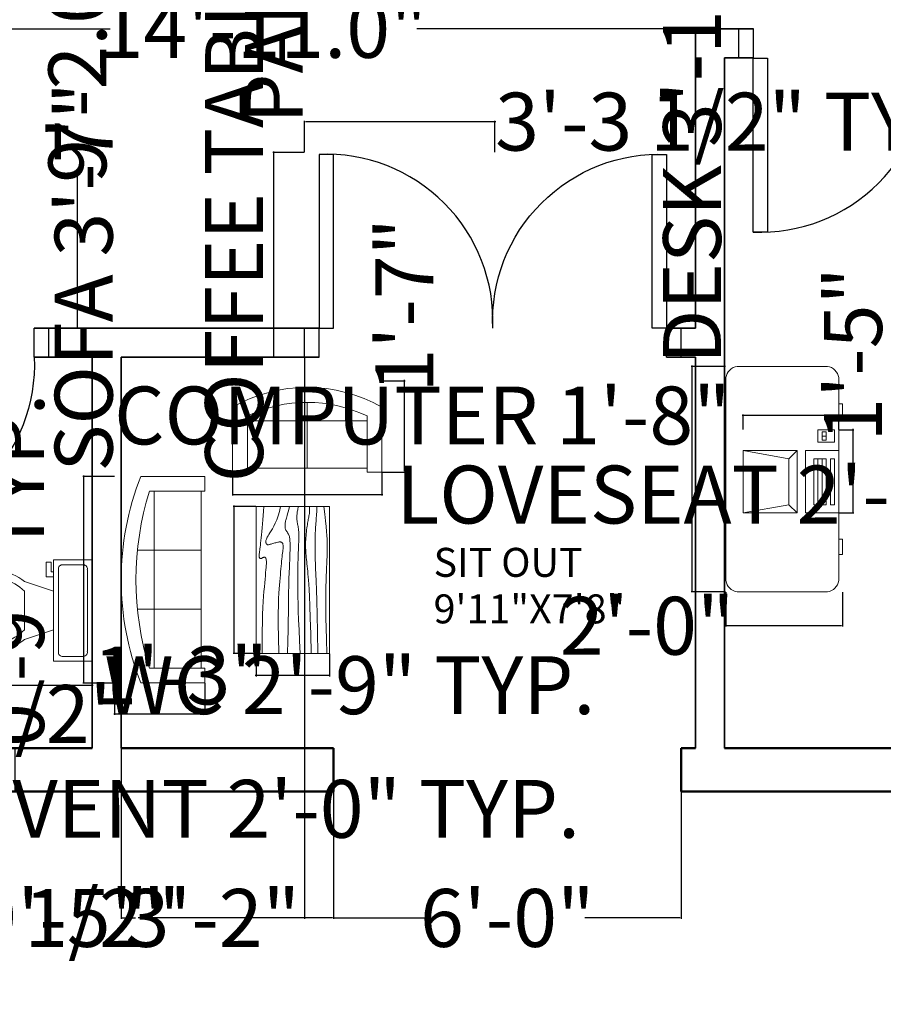
# Model space of a CAD drawing. Units: inches. Extents: x -52 to 472, y -40 to 644.
# Tile 2 of 6: x 71 to 250, y -40 to 164. Entities that reach past the tile are written whole.
import ezdxf

# ---------------------------------------------------------------- set-up
doc = ezdxf.new("R2010")
doc.units = ezdxf.units.IN
doc.header["$MEASUREMENT"] = 0
for name, color, linetype, lineweight in [('A-ANNO-DIMS', 7, 'Continuous', 13), ('A-ANNO-TEXT', 7, 'Continuous', 18), ('A-EQPM', 8, 'Continuous', 13), ('DOORS', 2, 'Continuous', 25), ('FURNITURE', 6, 'Continuous', 13), ('INNER WALL', 1, 'Continuous', 35), ('OUTER WALL', 1, 'Continuous', 50), ('S-PLUM', 151, 'Continuous', 18)]:
    doc.layers.add(name, color=color, linetype=linetype, lineweight=lineweight)
doc.styles.get("Standard").update_dxf_attribs({"font": 'arial.ttf'})
doc.dimstyles.get("Standard").update_dxf_attribs({"dimtxt": 12, "dimasz": 0.18, "dimexe": 0.18, "dimexo": 0.0625, "dimgap": 0.09, "dimtad": 0, "dimdec": 1, "dimzin": 0, "dimdsep": 46, "dimlunit": 3, "dimtxsty": 'Standard', "dimcen": 0.09, "dimadec": 0, "dimazin": 0, "dimtfac": 1, "dimtdec": 1, "dimtofl": 0, "dimtmove": 0, "dimatfit": 3, "dimfxl": 1, "dimtolj": 1, "dimtzin": 0, "dimarcsym": 0})

# ---------------------------------------------------------------- blocks, each defined once
blk = doc.blocks.new('Sofa - Roundback Loveseat 5 ft.')
for p, q in [((0, -32.44198), (0, -5.99998)), ((-24, -33.99998), (-24, -11.46958)), ((24.00004, -33.99998), (24.00004, -11.46958)), ((-23.9998, -13.38178), (23.99986, -13.38178)), ((-24, -32.44198), (24.00004, -32.44198))]:
    blk.add_line(p, q)
for points in [[(-24, -33.99998), (-30, -33.99998), (-30, -7.99998)], [(30.00004, -7.99998), (30.00004, -33.99998), (24.00004, -33.99998)]]:
    blk.add_lwpolyline(points)
for centre, radius, start, end in [((0, -60.24998), 60.24998, 60.13715, 119.8628), ((0, -61.38438), 55.38444, 64.32083, 115.6792)]:
    blk.add_arc(centre, radius, start, end)
blk = doc.blocks.new('Sofa - Roundback 7 ft.')
for p, q in [((-12.00002, -32.4421), (-12.00003, -6.5971)), ((11.99997, -32.4421), (11.99998, -6.5971)), ((-36.000027, -34), (-36.000027, -11.4696)), ((35.99998, -34), (35.99998, -11.4696)), ((-35.999844, -13.3819), (35.9998, -13.3819)), ((-36.000027, -32.4421), (35.99998, -32.4421))]:
    blk.add_line(p, q)
for points in [[(-36.000027, -34), (-42.000027, -34), (-42.000027, -8)], [(41.99998, -8), (41.99998, -34), (35.99998, -34)]]:
    blk.add_lwpolyline(points)
for centre, radius, start, end in [((0, -114.25), 114.25, 68.43141, 111.5686), ((-0.00001, -127.1968), 121.1968, 72.72033, 107.2797)]:
    blk.add_arc(centre, radius, start, end)
blk = doc.blocks.new('Table - Rectangular Woodgrain 60 x 30 in.')
for p, q in [((0, 0), (0, -30)), ((60, 0), (0, 0)), ((60, -30), (60, 0)), ((0, -30), (60, -30))]:
    blk.add_line(p, q)
for points in [[(0, -2.4), (4.8155, -2.418), (9.0302, -2.4688), (12.709, -2.5477), (15.9167, -2.65), (18.7181, -2.7711), (21.1781, -2.9063), (23.3616, -3.0508), (25.3333, -3.2), (27.1477, -3.3495), (28.8172, -3.4958), (30.3437, -3.636), (31.7291, -3.7667), (32.9756, -3.8849), (34.0849, -3.9875), (35.059, -4.0714), (35.9, -4.1334), (36.6114, -4.1711), (37.2041, -4.1854), (37.6906, -4.1779), (38.0833, -4.15), (38.3948, -4.1034), (38.6375, -4.0396), (38.8239, -3.9602), (38.9666, -3.8667), (39.0764, -3.7608), (39.1573, -3.6448), (39.2116, -3.521), (39.2416, -3.3917), (39.2498, -3.2593), (39.2385, -3.1261), (39.21, -2.9944), (39.1666, -2.8667), (39.111, -2.7447), (39.0468, -2.6281), (38.978, -2.5163), (38.9083, -2.4083), (38.8418, -2.3035), (38.7823, -2.201), (38.7337, -2.1001), (38.7, -2), (38.6844, -1.9003), (38.6875, -1.8021), (38.7094, -1.707), (38.75, -1.6167), (38.8094, -1.5326), (38.8875, -1.4563), (38.9844, -1.3893), (39.1, -1.3333), (39.2351, -1.2896), (39.3937, -1.2583), (39.5804, -1.2396), (39.8, -1.2333), (40.057, -1.2396), (40.3562, -1.2583), (40.7023, -1.2896), (41.1, -1.3333), (41.5547, -1.3895), (42.0755, -1.4573), (42.6721, -1.5361), (43.3542, -1.625), (44.1316, -1.7233), (45.014, -1.8302), (46.0114, -1.9449), (47.1333, -2.0667), (48.3862, -2.1947), (49.7625, -2.3281), (51.2513, -2.4663), (52.8416, -2.6083), (54.5226, -2.7535), (56.2833, -2.9011), (58.1127, -3.0501), (60, -3.2)], [(0, -9.2), (6.5759, -9.0858), (11.9385, -9.0365), (16.2527, -9.0418), (19.6833, -9.0917), (22.3952, -9.1759), (24.5531, -9.2844), (26.322, -9.4069), (27.8666, -9.5333), (29.3241, -9.6553), (30.7203, -9.7719), (32.0532, -9.8837), (33.3208, -9.9917), (34.5213, -10.0965), (35.6526, -10.199), (36.7128, -10.2999), (37.7, -10.4), (38.6129, -10.4996), (39.4531, -10.5969), (40.223, -10.6895), (40.925, -10.775), (41.5613, -10.8512), (42.1344, -10.9156), (42.6465, -10.966), (43.1, -11), (43.4976, -11.0158), (43.8437, -11.0136), (44.143, -10.9942), (44.4, -10.9583), (44.6195, -10.9069), (44.8062, -10.8406), (44.9648, -10.7603), (45.1, -10.6667), (45.2155, -10.5598), (45.3114, -10.4365), (45.3871, -10.2929), (45.4416, -10.125), (45.4743, -9.929), (45.4844, -9.7011), (45.4709, -9.4371), (45.4333, -9.1333), (45.3716, -8.7883), (45.2896, -8.4104), (45.1919, -8.0107), (45.0833, -7.6), (44.9685, -7.1893), (44.8521, -6.7896), (44.7388, -6.4117), (44.6333, -6.0667), (44.54, -5.7628), (44.4614, -5.4979), (44.4001, -5.2675), (44.3583, -5.0667), (44.3384, -4.8909), (44.3427, -4.7354), (44.3736, -4.5956), (44.4333, -4.4667), (44.5236, -4.3453), (44.6427, -4.2333), (44.7884, -4.1339), (44.9583, -4.05), (45.1501, -3.9849), (45.3614, -3.9417), (45.59, -3.9234), (45.8333, -3.9333), (46.0915, -3.9749), (46.3734, -4.0531), (46.6906, -4.1736), (47.0542, -4.3417), (47.4756, -4.5629), (47.9661, -4.8427), (48.5372, -5.1866), (49.2, -5.6), (49.9676, -6.0844), (50.8594, -6.625), (51.8965, -7.2031), (53.1, -7.8), (54.491, -8.3969), (56.0906, -8.975), (57.9199, -9.5156), (60, -10)], [(0, -12.8), (5.1847, -12.9322), (9.6213, -13.0323), (13.3963, -13.1059), (16.5958, -13.1583), (19.3063, -13.1952), (21.614, -13.2219), (23.6054, -13.2439), (25.3666, -13.2667), (26.9728, -13.2947), (28.4531, -13.3281), (29.8256, -13.3663), (31.1083, -13.4083), (32.3191, -13.4535), (33.476, -13.501), (34.597, -13.5501), (35.7, -13.6), (36.7984, -13.6497), (37.8875, -13.6979), (38.9578, -13.743), (40, -13.7833), (41.0047, -13.8174), (41.9625, -13.8438), (42.864, -13.8607), (43.7, -13.8667), (44.4631, -13.8604), (45.1552, -13.8417), (45.7801, -13.8104), (46.3416, -13.7667), (46.8439, -13.7104), (47.2906, -13.6417), (47.6858, -13.5604), (48.0333, -13.4667), (48.3375, -13.3608), (48.6042, -13.2448), (48.8396, -13.121), (49.05, -12.9917), (49.2417, -12.8593), (49.4208, -12.7261), (49.5937, -12.5944), (49.7667, -12.4667), (49.9452, -12.3451), (50.1323, -12.2313), (50.3303, -12.1268), (50.5416, -12.0333), (50.7686, -11.9524), (51.0135, -11.8854), (51.2788, -11.8341), (51.5666, -11.8), (51.8785, -11.7843), (52.2116, -11.7865), (52.562, -11.8059), (52.926, -11.8417), (53.2998, -11.8931), (53.6795, -11.9594), (54.0614, -12.0397), (54.4416, -12.1333), (54.8223, -12.2401), (55.2293, -12.3625), (55.6942, -12.5037), (56.2489, -12.6667), (56.9251, -12.8547), (57.7545, -13.0708), (58.7689, -13.3182), (60, -13.6)], [(0, -18), (5.124, -17.7273), (9.6609, -17.5057), (13.6705, -17.3303), (17.2125, -17.1958), (20.3467, -17.0973), (23.1328, -17.0297), (25.6307, -16.9878), (27.9, -16.9667), (29.9928, -16.9617), (31.9302, -16.9703), (33.7254, -16.9907), (35.3917, -17.0208), (36.9423, -17.0588), (38.3906, -17.1026), (39.7499, -17.1503), (41.0333, -17.2), (42.2519, -17.2496), (43.4073, -17.2969), (44.4986, -17.3395), (45.525, -17.375), (46.4858, -17.4012), (47.3802, -17.4156), (48.2074, -17.416), (48.9667, -17.4), (49.6583, -17.3662), (50.2872, -17.3167), (50.8595, -17.2547), (51.3812, -17.1833), (51.8584, -17.1057), (52.2971, -17.025), (52.7034, -16.9443), (53.0833, -16.8667), (53.443, -16.7951), (53.789, -16.7313), (54.128, -16.6768), (54.4666, -16.6334), (54.8115, -16.6024), (55.1693, -16.5854), (55.5465, -16.5841), (55.95, -16.6), (56.3828, -16.6337), (56.8346, -16.6823), (57.2915, -16.7418), (57.7396, -16.8084), (58.165, -16.878), (58.5539, -16.9469), (58.8924, -17.0111), (59.1666, -17.0667), (59.3679, -17.1107), (59.5078, -17.1438), (59.6032, -17.1675), (59.6708, -17.1833), (59.7275, -17.193), (59.7901, -17.1979), (59.8753, -17.1998), (60, -17.2)], [(0, -22.4), (8.0098, -22.2501), (14.4094, -22.1011), (19.4168, -21.9535), (23.25, -21.8083), (26.1269, -21.6663), (28.2656, -21.5281), (29.884, -21.3947), (31.2, -21.2667), (32.3967, -21.1448), (33.5172, -21.0292), (34.5697, -20.9198), (35.5625, -20.8167), (36.5037, -20.7198), (37.4015, -20.6292), (38.2642, -20.5448), (39.1, -20.4667), (39.9164, -20.3951), (40.7187, -20.3313), (41.5117, -20.2768), (42.3, -20.2333), (43.0883, -20.2024), (43.8812, -20.1854), (44.6836, -20.1841), (45.5, -20.2), (46.3328, -20.234), (47.1747, -20.2844), (48.0163, -20.3488), (48.8479, -20.425), (49.66, -20.5106), (50.4429, -20.6031), (51.1872, -20.7004), (51.8833, -20.8), (52.5246, -20.8999), (53.1166, -20.9995), (53.6681, -21.0983), (54.1875, -21.1958), (54.6834, -21.2919), (55.1646, -21.3859), (55.6394, -21.4777), (56.1167, -21.5667), (56.6028, -21.6515), (57.0961, -21.7266), (57.5929, -21.7852), (58.0896, -21.8208), (58.5823, -21.8268), (59.0674, -21.7964), (59.5412, -21.723), (60, -21.6)], [(0, -25.2), (8.6355, -25.0504), (15.7026, -24.9031), (21.4049, -24.7606), (25.9458, -24.625), (29.529, -24.4988), (32.3578, -24.3844), (34.6359, -24.284), (36.5667, -24.2), (38.3213, -24.1341), (39.9417, -24.0854), (41.437, -24.0523), (42.8167, -24.0333), (44.0901, -24.0268), (45.2667, -24.0313), (46.3557, -24.0451), (47.3667, -24.0667), (48.309, -24.0947), (49.1928, -24.1287), (50.0284, -24.168), (50.826, -24.2125), (51.5959, -24.2617), (52.3483, -24.3151), (53.0935, -24.3725), (53.8417, -24.4334), (54.6009, -24.497), (55.3699, -24.561), (56.1454, -24.6226), (56.9239, -24.6792), (57.7021, -24.7279), (58.4764, -24.7662), (59.2435, -24.7911), (60, -24.8)], [(0, -28.8), (5.6867, -28.6681), (10.45, -28.5698), (14.407, -28.5012), (17.675, -28.4584), (20.3711, -28.4374), (22.6125, -28.4344), (24.5164, -28.4455), (26.2, -28.4667), (27.762, -28.4947), (29.2276, -28.5281), (30.6033, -28.5663), (31.8958, -28.6084), (33.1118, -28.6535), (34.2578, -28.7011), (35.3405, -28.7501), (36.3666, -28.8), (37.3443, -28.8497), (38.288, -28.8974), (39.2137, -28.9412), (40.1375, -28.9792), (41.0753, -29.0093), (42.0432, -29.0297), (43.0572, -29.0384), (44.1333, -29.0333), (45.2936, -29.0114), (46.5843, -28.9641), (48.0579, -28.8816), (49.7666, -28.7542), (51.7629, -28.5721), (54.0989, -28.3255), (56.8272, -28.0048), (60, -27.6)]]:
    blk.add_lwpolyline(points)
blk = doc.blocks.new('Toilet - top')
for p, q in [((9.5, -6), (9.5, -2)), ((-8, -8.5), (-8, -8)), ((-7, -8), (-7, -9.5)), ((-4, -8), (-6, -14)), ((4, -8), (6, -14)), ((-10, -8.5), (-8, -8.5)), ((-10, -9.5), (-10, -8.5)), ((-7, -9.5), (-10, -9.5)), ((4, -14), (-4, -14))]:
    blk.add_line(p, q)
blk.add_lwpolyline([(10.5, -8), (10.5, 0), (-10.5, 0), (-10.5, -8)], close=True)
for points in [[(-9.5, -2), (-9.5, -6)], [(8.5, -1), (-8.5, -1)], [(-8.5, -7), (8.5, -7)]]:
    blk.add_lwpolyline(points)
for centre, radius, start, end in [((-8.62, -1.88), 0.884, 81.8699, 188.1301), ((8.62, -1.88), 0.884, 351.8699, 98.1301), ((-8.62, -6.12), 0.884, 171.8699, 278.1301), ((8.62, -6.12), 0.884, 261.8699, 8.1301), ((3.52, -21.58), 12.17, 141.4691, 247.9714), ((4.2, -21.82), 11.33, 136.3677, 238.9468), ((-3.52, -21.58), 12.17, 292.0284, 38.5307), ((-4.2, -21.82), 11.33, 301.053, 43.6321), ((0, -27.88), 4, 245.7318, 294.2682), ((0, -29), 4, 254.8605, 285.1395)]:
    blk.add_arc(centre, radius, start, end)
blk = doc.blocks.new('*D16')
at = {"layer": 'A-ANNO-DIMS', "color": 0, "lineweight": -2, "transparency": 16777216}
for p, q in [((88.57, 210.33), (82.89, 210.33)), ((83.07, 210.15), (83.07, 178.36)), ((83.07, 100.51), (83.07, 132.3)), ((88.57, 100.33), (82.89, 100.33))]:
    blk.add_line(p, q, dxfattribs=at)
at = {"layer": 'A-ANNO-DIMS', "color": 0, "transparency": 16777216}
for points in [[(83.04, 210.15), (83.1, 210.15), (83.07, 210.33)], [(83.04, 100.51), (83.1, 100.51), (83.07, 100.33)]]:
    blk.add_solid(points, dxfattribs=at)
at = {"layer": 'Defpoints', "color": 0, "transparency": 16777216}
for p in [(88.63, 210.33), (83.07, 100.33), (88.63, 100.33)]:
    blk.add_point(p, dxfattribs=at)
at = {"layer": 'A-ANNO-DIMS', "color": 0, "transparency": 16777216, "insert": (83.07, 155.33), "char_height": 12, "attachment_point": 5, "rotation": 90}
blk.add_mtext('\\A1;9\'-2.0"', dxfattribs=at)
blk = doc.blocks.new('*D17')
at = {"layer": 'A-ANNO-DIMS', "color": 0, "lineweight": -2, "transparency": 16777216}
for p, q in [((32.13, 162.39), (32.13, 162.51)), ((32.31, 162.33), (89.84, 162.33)), ((210.95, 162.33), (153.42, 162.33)), ((211.13, 162.39), (211.13, 162.51))]:
    blk.add_line(p, q, dxfattribs=at)
at = {"layer": 'A-ANNO-DIMS', "color": 0, "transparency": 16777216}
for points in [[(32.31, 162.36), (32.31, 162.3), (32.13, 162.33)], [(210.95, 162.36), (210.95, 162.3), (211.13, 162.33)]]:
    blk.add_solid(points, dxfattribs=at)
at = {"layer": 'Defpoints', "color": 0, "transparency": 16777216}
for p in [(32.13, 162.33), (32.13, 162.33), (211.13, 162.33)]:
    blk.add_point(p, dxfattribs=at)
at = {"layer": 'A-ANNO-DIMS', "color": 0, "transparency": 16777216, "insert": (121.63, 162.33), "char_height": 12, "attachment_point": 5}
blk.add_mtext('\\A1;14\'-11.0"', dxfattribs=at)
blk = doc.blocks.new('Computer Terminal')
for p, q in [((-10, 11.5), (5, 11.5)), ((-8, 0.5), (-10, 11.5)), ((-10, -1.5), (-10, 11.5)), ((5, 11.5), (3, 0.5)), ((5, 11.5), (5, -1.5)), ((-10, -1.5), (-8, 0.5)), ((3, 0.5), (-8, 0.5)), ((3, 0.5), (5, -1.5)), ((5, -1.5), (-10, -1.5)), ((-10, -11.5), (-10, -3.5)), ((-10, -3.5), (5, -3.5)), ((5, -3.5), (5, -11.5)), ((-8, -5.5), (-8, -8.5)), ((3, -5.5), (-8, -5.5)), ((3, -6.5), (-8, -6.5)), ((3, -8.5), (3, -5.5)), ((10, -6.5), (7, -6.5)), ((7, -6.5), (7, -10.5)), ((10, -10.5), (10, -6.5)), ((-8, -7.5), (3, -7.5)), ((-8, -8.5), (3, -8.5)), ((9.5, -7.5), (7.5, -7.5)), ((7.5, -7.5), (7.5, -8.5)), ((7.5, -8.5), (9.5, -8.5)), ((8.5, -7.5), (8.5, -8.5)), ((9.5, -8.5), (9.5, -7.5)), ((5, -11.5), (-10, -11.5)), ((-8, -9.5), (-8, -10.5)), ((3, -9.5), (-8, -9.5)), ((-8, -10.5), (3, -10.5)), ((3, -10.5), (3, -9.5)), ((7, -10.5), (10, -10.5))]:
    blk.add_line(p, q)
blk = doc.blocks.new('Desk - 30 x 60 in.')
for p, q in [((-26.999995, 0), (26.999995, 0)), ((-29.999995, -27), (-29.999995, -3)), ((29.999995, -3), (29.999995, -27)), ((26.999995, -30), (-26.999995, -30)), ((-20.000005, -30), (-20.000005, -31)), ((-20.000005, -31), (-16.000005, -31)), ((-16.000005, -31), (-16.000005, -30)), ((15.999995, -31), (15.999995, -30)), ((19.999995, -31), (15.999995, -31)), ((19.999995, -30), (19.999995, -31))]:
    blk.add_line(p, q)
for centre, start, end in [((-26.499995, -3.5), 98.1301, 171.8699), ((26.499995, -3.5), 8.130102, 81.8699), ((-26.499995, -26.5), 188.1301, 261.8699), ((26.499995, -26.5), 278.1301, 351.8699)]:
    blk.add_arc(centre, 3.535534, start, end)
blk = doc.blocks.new('DOOR-36IN-SINGLE')
for p, q in [((0, 6), (0, 0)), ((3, 6), (3, 0)), ((39, 6), (39, 0)), ((42, 6), (42, 0))]:
    blk.add_line(p, q)
blk.add_lwpolyline([(3, 6), (6, 6), (6, 42), (3, 42)], close=True)
blk.add_arc((4.5, 7.5), 34.53, 357.5104, 92.4896)
blk = doc.blocks.new('DOOR-36IN-PAIRED-LEAF')
for p, q in [((0, 0), (0, 6)), ((3, 0), (3, 6))]:
    blk.add_line(p, q)
blk.add_lwpolyline([(3, 6), (6, 6), (6, 42), (3, 42)], close=True)
blk.add_arc((4.5, 7.5), 34.53, 357.5104, 92.4896)
blk = doc.blocks.new('*D40')
at = {"layer": 'A-ANNO-DIMS', "color": 0, "lineweight": -2, "transparency": 16777216}
for p, q in [((220.99, 82.23), (220.81, 82.23)), ((220.99, 79.32), (220.99, 82.41)), ((240.62, 82.23), (221.17, 82.23)), ((240.8, 79.32), (240.8, 82.41))]:
    blk.add_line(p, q, dxfattribs=at)
at = {"layer": 'A-ANNO-DIMS', "color": 0, "transparency": 16777216}
for points in [[(221.17, 82.26), (221.17, 82.2), (220.99, 82.23)], [(240.62, 82.26), (240.62, 82.2), (240.8, 82.23)]]:
    blk.add_solid(points, dxfattribs=at)
at = {"layer": 'Defpoints', "color": 0, "transparency": 16777216}
for p in [(220.99, 82.23), (220.99, 79.26), (240.8, 79.26)]:
    blk.add_point(p, dxfattribs=at)
at = {"layer": 'A-ANNO-DIMS', "color": 0, "transparency": 16777216, "insert": (154.55, 82.23), "char_height": 12, "attachment_point": 5}
blk.add_mtext('\\A1;COMPUTER 1\'-8"', dxfattribs=at)
blk = doc.blocks.new('*D41')
at = {"layer": 'A-ANNO-DIMS', "color": 0, "lineweight": -2, "transparency": 16777216}
for p, q in [((240.86, 79.26), (243.95, 79.26)), ((243.77, 79.26), (243.77, 79.44)), ((243.77, 62.21), (243.77, 79.08)), ((240.86, 62.03), (243.95, 62.03))]:
    blk.add_line(p, q, dxfattribs=at)
at = {"layer": 'A-ANNO-DIMS', "color": 0, "transparency": 16777216}
for points in [[(243.74, 79.08), (243.8, 79.08), (243.77, 79.26)], [(243.74, 62.21), (243.8, 62.21), (243.77, 62.03)]]:
    blk.add_solid(points, dxfattribs=at)
at = {"layer": 'Defpoints', "color": 0, "transparency": 16777216}
for p in [(240.8, 79.26), (243.77, 79.26), (240.8, 62.03)]:
    blk.add_point(p, dxfattribs=at)
at = {"layer": 'A-ANNO-DIMS', "color": 0, "transparency": 16777216, "insert": (243.77, 94.91), "char_height": 12, "attachment_point": 5, "rotation": 90}
blk.add_mtext('\\A1;1\'-5"', dxfattribs=at)
blk = doc.blocks.new('*D44')
at = {"layer": 'A-ANNO-DIMS', "color": 0, "lineweight": -2, "transparency": 16777216}
for p, q in [((217.37, 92.41), (210.24, 92.41)), ((210.42, 92.41), (210.42, 92.59)), ((210.42, 45.85), (210.42, 92.23)), ((217.37, 45.67), (210.24, 45.67))]:
    blk.add_line(p, q, dxfattribs=at)
at = {"layer": 'A-ANNO-DIMS', "color": 0, "transparency": 16777216}
for points in [[(210.39, 92.23), (210.45, 92.23), (210.42, 92.41)], [(210.39, 45.85), (210.45, 45.85), (210.42, 45.67)]]:
    blk.add_solid(points, dxfattribs=at)
at = {"layer": 'Defpoints', "color": 0, "transparency": 16777216}
for p in [(210.42, 92.41), (217.43, 92.41), (217.43, 45.67)]:
    blk.add_point(p, dxfattribs=at)
at = {"layer": 'A-ANNO-DIMS', "color": 0, "transparency": 16777216, "insert": (210.42, 152.12), "char_height": 12, "attachment_point": 5, "rotation": 90}
blk.add_mtext('\\A1;DESK 3\'-10 1/2"', dxfattribs=at)
blk = doc.blocks.new('*D45')
at = {"layer": 'A-ANNO-DIMS', "color": 0, "lineweight": -2, "transparency": 16777216}
for p, q in [((217.43, 45.61), (217.43, 38.48)), ((241.58, 45.61), (241.58, 38.48)), ((217.43, 38.66), (217.25, 38.66)), ((241.4, 38.66), (217.61, 38.66))]:
    blk.add_line(p, q, dxfattribs=at)
at = {"layer": 'A-ANNO-DIMS', "color": 0, "transparency": 16777216}
for points in [[(217.61, 38.69), (217.61, 38.63), (217.43, 38.66)], [(241.4, 38.69), (241.4, 38.63), (241.58, 38.66)]]:
    blk.add_solid(points, dxfattribs=at)
at = {"layer": 'Defpoints', "color": 0, "transparency": 16777216}
for p in [(217.43, 45.67), (241.58, 45.67), (217.43, 38.66)]:
    blk.add_point(p, dxfattribs=at)
at = {"layer": 'A-ANNO-DIMS', "color": 0, "transparency": 16777216, "insert": (201.11, 38.66), "char_height": 12, "attachment_point": 5}
blk.add_mtext('\\A1;2\'-0"', dxfattribs=at)
blk = doc.blocks.new('*D46')
at = {"layer": 'A-ANNO-DIMS', "color": 0, "lineweight": -2, "transparency": 16777216}
for p, q in [((53.09, 31.25), (53.09, 26.17)), ((86.13, 31.25), (86.13, 26.17)), ((53.27, 26.35), (85.95, 26.35)), ((86.13, 26.35), (86.31, 26.35))]:
    blk.add_line(p, q, dxfattribs=at)
at = {"layer": 'A-ANNO-DIMS', "color": 0, "transparency": 16777216}
for points in [[(53.27, 26.38), (53.27, 26.32), (53.09, 26.35)], [(85.95, 26.38), (85.95, 26.32), (86.13, 26.35)]]:
    blk.add_solid(points, dxfattribs=at)
at = {"layer": 'Defpoints', "color": 0, "transparency": 16777216}
for p in [(53.09, 31.31), (86.13, 31.31), (86.13, 26.35)]:
    blk.add_point(p, dxfattribs=at)
at = {"layer": 'A-ANNO-DIMS', "color": 0, "transparency": 16777216, "insert": (139.51, 26.35), "char_height": 12, "attachment_point": 5}
blk.add_mtext('\\A1;WC 2\'-9" TYP.', dxfattribs=at)
blk = doc.blocks.new('*D48')
at = {"layer": 'A-ANNO-DIMS', "color": 0, "lineweight": -2, "transparency": 16777216}
for p, q in [((42.57, 4.27), (42.57, 0.55)), ((66.57, 4.27), (66.57, 0.55)), ((42.75, 0.73), (66.39, 0.73)), ((66.57, 0.73), (66.75, 0.73))]:
    blk.add_line(p, q, dxfattribs=at)
at = {"layer": 'A-ANNO-DIMS', "color": 0, "transparency": 16777216}
for points in [[(42.75, 0.76), (42.75, 0.7), (42.57, 0.73)], [(66.39, 0.76), (66.39, 0.7), (66.57, 0.73)]]:
    blk.add_solid(points, dxfattribs=at)
at = {"layer": 'Defpoints', "color": 0, "transparency": 16777216}
for p in [(42.57, 4.33), (66.57, 4.33), (66.57, 0.73)]:
    blk.add_point(p, dxfattribs=at)
at = {"layer": 'A-ANNO-DIMS', "color": 0, "transparency": 16777216, "insert": (128.4, 0.73), "char_height": 12, "attachment_point": 5}
blk.add_mtext('\\A1;VENT 2\'-0" TYP.', dxfattribs=at)
blk = doc.blocks.new('*D49')
at = {"layer": 'A-ANNO-DIMS', "color": 0, "lineweight": -2, "transparency": 16777216}
for p, q in [((66.63, 13.33), (70.35, 13.33)), ((70.17, 13.33), (70.17, 13.51)), ((70.17, 4.51), (70.17, 13.15)), ((66.63, 4.33), (70.35, 4.33))]:
    blk.add_line(p, q, dxfattribs=at)
at = {"layer": 'A-ANNO-DIMS', "color": 0, "transparency": 16777216}
for points in [[(70.14, 13.15), (70.2, 13.15), (70.17, 13.33)], [(70.14, 4.51), (70.2, 4.51), (70.17, 4.33)]]:
    blk.add_solid(points, dxfattribs=at)
at = {"layer": 'Defpoints', "color": 0, "transparency": 16777216}
for p in [(66.57, 13.33), (70.17, 13.33), (66.57, 4.33)]:
    blk.add_point(p, dxfattribs=at)
at = {"layer": 'A-ANNO-DIMS', "color": 0, "transparency": 16777216, "insert": (70.17, 50.17), "char_height": 12, "attachment_point": 5, "rotation": 90}
blk.add_mtext('\\A1;0\'-9" TYP.', dxfattribs=at)
blk = doc.blocks.new('*D52')
at = {"layer": 'A-ANNO-DIMS', "color": 0, "lineweight": -2, "transparency": 16777216}
for p, q in [((130.07, 136.75), (123.59, 136.75)), ((123.77, 136.75), (123.77, 136.93)), ((123.77, 94.51), (123.77, 136.57)), ((130.07, 94.33), (123.59, 94.33))]:
    blk.add_line(p, q, dxfattribs=at)
at = {"layer": 'A-ANNO-DIMS', "color": 0, "transparency": 16777216}
for points in [[(123.74, 136.57), (123.8, 136.57), (123.77, 136.75)], [(123.74, 94.51), (123.8, 94.51), (123.77, 94.33)]]:
    blk.add_solid(points, dxfattribs=at)
at = {"layer": 'Defpoints', "color": 0, "transparency": 16777216}
for p in [(123.77, 136.75), (130.13, 136.75), (130.13, 94.33)]:
    blk.add_point(p, dxfattribs=at)
at = {"layer": 'A-ANNO-DIMS', "color": 0, "transparency": 16777216, "insert": (123.77, 244.1), "char_height": 12, "attachment_point": 5, "rotation": 90}
blk.add_mtext('\\A1;PAIRED LEAF 3\'-6 1/2" TYP.', dxfattribs=at)
blk = doc.blocks.new('*D53')
at = {"layer": 'A-ANNO-DIMS', "color": 0, "lineweight": -2, "transparency": 16777216}
for p, q in [((130.13, 136.81), (130.13, 143.29)), ((130.31, 143.11), (169.37, 143.11)), ((169.55, 136.81), (169.55, 143.29)), ((169.55, 143.11), (169.73, 143.11))]:
    blk.add_line(p, q, dxfattribs=at)
at = {"layer": 'A-ANNO-DIMS', "color": 0, "transparency": 16777216}
for points in [[(130.31, 143.14), (130.31, 143.08), (130.13, 143.11)], [(169.37, 143.14), (169.37, 143.08), (169.55, 143.11)]]:
    blk.add_solid(points, dxfattribs=at)
at = {"layer": 'Defpoints', "color": 0, "transparency": 16777216}
for p in [(169.55, 143.11), (130.13, 136.75), (169.55, 136.75)]:
    blk.add_point(p, dxfattribs=at)
at = {"layer": 'A-ANNO-DIMS', "color": 0, "transparency": 16777216, "insert": (220.37, 143.11), "char_height": 12, "attachment_point": 5}
blk.add_mtext('\\A1;3\'-3 1/2" TYP.', dxfattribs=at)
blk = doc.blocks.new('*D56')
at = {"layer": 'A-ANNO-DIMS', "color": 0, "lineweight": -2, "transparency": 16777216}
for p, q in [((115.19, 70.43), (115.19, 65.67)), ((146.16, 70.43), (146.16, 65.67)), ((115.37, 65.85), (145.98, 65.85)), ((146.16, 65.85), (146.34, 65.85))]:
    blk.add_line(p, q, dxfattribs=at)
at = {"layer": 'A-ANNO-DIMS', "color": 0, "transparency": 16777216}
for points in [[(115.37, 65.88), (115.37, 65.82), (115.19, 65.85)], [(145.98, 65.88), (145.98, 65.82), (146.16, 65.85)]]:
    blk.add_solid(points, dxfattribs=at)
at = {"layer": 'Defpoints', "color": 0, "transparency": 16777216}
for p in [(115.19, 70.49), (146.16, 70.49), (146.16, 65.85)]:
    blk.add_point(p, dxfattribs=at)
at = {"layer": 'A-ANNO-DIMS', "color": 0, "transparency": 16777216, "insert": (208.7, 65.85), "char_height": 12, "attachment_point": 5}
blk.add_mtext('\\A1;LOVESEAT 2\'-7"', dxfattribs=at)
blk = doc.blocks.new('*D57')
at = {"layer": 'A-ANNO-DIMS', "color": 0, "lineweight": -2, "transparency": 16777216}
for p, q in [((146.23, 89.42), (150.99, 89.42)), ((150.81, 89.42), (150.81, 89.6)), ((150.81, 70.67), (150.81, 89.24)), ((146.23, 70.49), (150.99, 70.49))]:
    blk.add_line(p, q, dxfattribs=at)
at = {"layer": 'A-ANNO-DIMS', "color": 0, "transparency": 16777216}
for points in [[(150.78, 89.24), (150.84, 89.24), (150.81, 89.42)], [(150.78, 70.67), (150.84, 70.67), (150.81, 70.49)]]:
    blk.add_solid(points, dxfattribs=at)
at = {"layer": 'Defpoints', "color": 0, "transparency": 16777216}
for p in [(146.16, 89.42), (150.81, 89.42), (146.16, 70.49)]:
    blk.add_point(p, dxfattribs=at)
at = {"layer": 'A-ANNO-DIMS', "color": 0, "transparency": 16777216, "insert": (150.81, 105.08), "char_height": 12, "attachment_point": 5, "rotation": 90}
blk.add_mtext('\\A1;1\'-7"', dxfattribs=at)
blk = doc.blocks.new('*D58')
at = {"layer": 'A-ANNO-DIMS', "color": 0, "lineweight": -2, "transparency": 16777216}
for p, q in [((90.73, 69.61), (84.19, 69.61)), ((84.37, 69.61), (84.37, 69.79)), ((84.37, 26.98), (84.37, 69.43)), ((90.73, 26.8), (84.19, 26.8))]:
    blk.add_line(p, q, dxfattribs=at)
at = {"layer": 'A-ANNO-DIMS', "color": 0, "transparency": 16777216}
for points in [[(84.34, 69.43), (84.4, 69.43), (84.37, 69.61)], [(84.34, 26.98), (84.4, 26.98), (84.37, 26.8)]]:
    blk.add_solid(points, dxfattribs=at)
at = {"layer": 'Defpoints', "color": 0, "transparency": 16777216}
for p in [(84.37, 69.61), (90.79, 69.61), (90.79, 26.8)]:
    blk.add_point(p, dxfattribs=at)
at = {"layer": 'A-ANNO-DIMS', "color": 0, "transparency": 16777216, "insert": (84.37, 110.95), "char_height": 12, "attachment_point": 5, "rotation": 90}
blk.add_mtext('\\A1;SOFA 3\'-7"', dxfattribs=at)
blk = doc.blocks.new('*D59')
at = {"layer": 'A-ANNO-DIMS', "color": 0, "lineweight": -2, "transparency": 16777216}
for p, q in [((90.79, 26.74), (90.79, 20.2)), ((109.47, 26.74), (109.47, 20.2)), ((90.79, 20.38), (90.61, 20.38)), ((109.29, 20.38), (90.97, 20.38))]:
    blk.add_line(p, q, dxfattribs=at)
at = {"layer": 'A-ANNO-DIMS', "color": 0, "transparency": 16777216}
for points in [[(90.97, 20.41), (90.97, 20.35), (90.79, 20.38)], [(109.29, 20.41), (109.29, 20.35), (109.47, 20.38)]]:
    blk.add_solid(points, dxfattribs=at)
at = {"layer": 'Defpoints', "color": 0, "transparency": 16777216}
for p in [(90.79, 26.8), (109.47, 26.8), (90.79, 20.38)]:
    blk.add_point(p, dxfattribs=at)
at = {"layer": 'A-ANNO-DIMS', "color": 0, "transparency": 16777216, "insert": (61.15, 20.38), "char_height": 12, "attachment_point": 5}
blk.add_mtext('\\A1;1\'-6 1/2"', dxfattribs=at)
blk = doc.blocks.new('*D60')
at = {"layer": 'A-ANNO-DIMS', "color": 0, "lineweight": -2, "transparency": 16777216}
for p, q in [((120.04, 63.4), (115.35, 63.4)), ((115.53, 63.4), (115.53, 63.58)), ((115.53, 33.11), (115.53, 63.22)), ((120.04, 32.93), (115.35, 32.93))]:
    blk.add_line(p, q, dxfattribs=at)
at = {"layer": 'A-ANNO-DIMS', "color": 0, "transparency": 16777216}
for points in [[(115.5, 63.22), (115.56, 63.22), (115.53, 63.4)], [(115.5, 33.11), (115.56, 33.11), (115.53, 32.93)]]:
    blk.add_solid(points, dxfattribs=at)
at = {"layer": 'Defpoints', "color": 0, "transparency": 16777216}
for p in [(115.53, 63.4), (120.1, 63.4), (120.1, 32.93)]:
    blk.add_point(p, dxfattribs=at)
at = {"layer": 'A-ANNO-DIMS', "color": 0, "transparency": 16777216, "insert": (115.53, 158.74), "char_height": 12, "attachment_point": 5, "rotation": 90}
blk.add_mtext('\\A1;COFFEE TABLE 2\'-6 1/2"', dxfattribs=at)
blk = doc.blocks.new('*D61')
at = {"layer": 'A-ANNO-DIMS', "color": 0, "lineweight": -2, "transparency": 16777216}
for p, q in [((120.1, 32.87), (120.1, 28.18)), ((135.33, 32.87), (135.33, 28.18)), ((120.1, 28.36), (119.92, 28.36)), ((135.15, 28.36), (120.28, 28.36))]:
    blk.add_line(p, q, dxfattribs=at)
at = {"layer": 'A-ANNO-DIMS', "color": 0, "transparency": 16777216}
for points in [[(120.28, 28.39), (120.28, 28.33), (120.1, 28.36)], [(135.15, 28.39), (135.15, 28.33), (135.33, 28.36)]]:
    blk.add_solid(points, dxfattribs=at)
at = {"layer": 'Defpoints', "color": 0, "transparency": 16777216}
for p in [(120.1, 32.93), (135.33, 32.93), (120.1, 28.36)]:
    blk.add_point(p, dxfattribs=at)
at = {"layer": 'A-ANNO-DIMS', "color": 0, "transparency": 16777216, "insert": (104.44, 28.36), "char_height": 12, "attachment_point": 5}
blk.add_mtext('\\A1;1\'-3"', dxfattribs=at)
blk = doc.blocks.new('*D74')
at = {"layer": 'A-ANNO-DIMS', "color": 0, "lineweight": -2, "transparency": 16777216}
for p, q in [((136.13, 4.27), (136.13, -22.05)), ((208.13, 4.27), (208.13, -22.05)), ((136.31, -21.87), (156.06, -21.87)), ((207.95, -21.87), (188.2, -21.87))]:
    blk.add_line(p, q, dxfattribs=at)
at = {"layer": 'A-ANNO-DIMS', "color": 0, "transparency": 16777216}
for points in [[(136.31, -21.84), (136.31, -21.9), (136.13, -21.87)], [(207.95, -21.84), (207.95, -21.9), (208.13, -21.87)]]:
    blk.add_solid(points, dxfattribs=at)
at = {"layer": 'Defpoints', "color": 0, "transparency": 16777216}
for p in [(136.13, 4.33), (208.13, 4.33), (208.13, -21.87)]:
    blk.add_point(p, dxfattribs=at)
at = {"layer": 'A-ANNO-DIMS', "color": 0, "transparency": 16777216, "insert": (172.13, -21.87), "char_height": 12, "attachment_point": 5}
blk.add_mtext('\\A1;6\'-0"', dxfattribs=at)
blk = doc.blocks.new('*D75')
at = {"layer": 'A-ANNO-DIMS', "color": 0, "lineweight": -2, "transparency": 16777216}
for p, q in [((23.13, 4.27), (23.13, -22.05)), ((136.13, 4.27), (136.13, -22.05)), ((23.31, -21.87), (63.59, -21.87)), ((135.95, -21.87), (95.67, -21.87))]:
    blk.add_line(p, q, dxfattribs=at)
at = {"layer": 'A-ANNO-DIMS', "color": 0, "transparency": 16777216}
for points in [[(23.31, -21.84), (23.31, -21.9), (23.13, -21.87)], [(135.95, -21.84), (135.95, -21.9), (136.13, -21.87)]]:
    blk.add_solid(points, dxfattribs=at)
at = {"layer": 'Defpoints', "color": 0, "transparency": 16777216}
for p in [(23.13, 4.33), (136.13, 4.33), (136.13, -21.87)]:
    blk.add_point(p, dxfattribs=at)
at = {"layer": 'A-ANNO-DIMS', "color": 0, "transparency": 16777216, "insert": (79.63, -21.87), "char_height": 12, "attachment_point": 5}
blk.add_mtext('\\A1;9\'-5"', dxfattribs=at)
blk = doc.blocks.new('*D76')
at = {"layer": 'A-ANNO-DIMS', "color": 0, "lineweight": -2, "transparency": 16777216}
for p, q in [((23.13, 4.27), (23.13, -22.05)), ((42.57, 4.27), (42.57, -22.05)), ((23.31, -21.87), (42.39, -21.87)), ((42.57, -21.87), (42.75, -21.87))]:
    blk.add_line(p, q, dxfattribs=at)
at = {"layer": 'A-ANNO-DIMS', "color": 0, "transparency": 16777216}
for points in [[(23.31, -21.84), (23.31, -21.9), (23.13, -21.87)], [(42.39, -21.84), (42.39, -21.9), (42.57, -21.87)]]:
    blk.add_solid(points, dxfattribs=at)
at = {"layer": 'Defpoints', "color": 0, "transparency": 16777216}
for p in [(23.13, 4.33), (42.57, 4.33), (42.57, -21.87)]:
    blk.add_point(p, dxfattribs=at)
at = {"layer": 'A-ANNO-DIMS', "color": 0, "transparency": 16777216, "insert": (72.2, -21.87), "char_height": 12, "attachment_point": 5}
blk.add_mtext('\\A1;1\'-7 1/2"', dxfattribs=at)
blk = doc.blocks.new('*D82')
at = {"layer": 'A-ANNO-DIMS', "color": 0, "lineweight": -2, "transparency": 16777216}
for p, q in [((92.13, 94.27), (92.13, -22.05)), ((130.13, 94.27), (130.13, -22.05)), ((92.31, -21.87), (95.1, -21.87)), ((129.95, -21.87), (127.17, -21.87))]:
    blk.add_line(p, q, dxfattribs=at)
at = {"layer": 'A-ANNO-DIMS', "color": 0, "transparency": 16777216}
for points in [[(92.31, -21.84), (92.31, -21.9), (92.13, -21.87)], [(129.95, -21.84), (129.95, -21.9), (130.13, -21.87)]]:
    blk.add_solid(points, dxfattribs=at)
at = {"layer": 'Defpoints', "color": 0, "transparency": 16777216}
for p in [(92.13, 94.33), (130.13, 94.33), (92.13, -21.87)]:
    blk.add_point(p, dxfattribs=at)
at = {"layer": 'A-ANNO-DIMS', "color": 0, "transparency": 16777216, "insert": (111.13, -21.87), "char_height": 12, "attachment_point": 5}
blk.add_mtext('\\A1;3\'-2"', dxfattribs=at)

msp = doc.modelspace()

# ---------------------------------------------------------------- linework, layer by layer
at = {"layer": 'DOORS'}
for p, q in [((220.13, 156.33), (220.13, 162.33)), ((223.13, 156.33), (223.13, 162.33))]:
    msp.add_line(p, q, dxfattribs=at)
msp.add_lwpolyline([(223.05, 156.24), (226.05, 156.24), (226.05, 120.24), (223.05, 120.24)], close=True, dxfattribs=at)
msp.add_arc((224.55, 154.83), 34.62, 267.5165, 2.4828, dxfattribs=at)
at = {"layer": 'INNER WALL'}
for p, q in [((211.13, 162.33), (223.13, 162.33)), ((211.13, 162.33), (211.13, 100.33)), ((217.13, 156.33), (223.13, 156.33)), ((217.13, 156.33), (217.13, 13.33)), ((133.13, 100.33), (74.13, 100.33)), ((211.13, 100.33), (205.13, 100.33)), ((86.13, 94.33), (74.13, 94.33)), ((86.13, 94.33), (86.13, 13.33)), ((92.13, 94.33), (92.13, 13.33)), ((133.13, 94.33), (92.13, 94.33)), ((211.13, 94.33), (205.13, 94.33)), ((211.13, 94.33), (211.13, 13.33))]:
    msp.add_line(p, q, dxfattribs=at)
at = {"layer": 'OUTER WALL'}
for p, q in [((32.13, 13.33), (86.13, 13.33)), ((92.13, 13.33), (136.13, 13.33)), ((136.13, 4.33), (136.13, 13.33)), ((208.13, 13.33), (211.13, 13.33)), ((208.13, 4.33), (208.13, 13.33)), ((217.13, 13.33), (344.13, 13.33))]:
    msp.add_line(p, q, dxfattribs=at)
msp.add_lwpolyline([(208.13, 4.33), (353.13, 4.33), (353.13, 482.33), (23.13, 482.33), (23.13, 4.33), (136.13, 4.33)], dxfattribs=at)

# ---------------------------------------------------------------- block references
at = {"layer": 'A-EQPM', "xscale": 0.8612085498935265, "yscale": 0.8612085498935265, "zscale": 0.8612085498935265, "rotation": 90}
msp.add_blockref('Computer Terminal', (230.9, 70.64), dxfattribs=at)
at = {"layer": 'DOORS'}
msp.add_blockref('DOOR-36IN-PAIRED-LEAF', (130.13, 94.33), dxfattribs=at)
at = {"layer": 'DOORS', "extrusion": (0, 0, -1), "zscale": -1}
msp.add_blockref('DOOR-36IN-PAIRED-LEAF', (-208.13, 94.33), dxfattribs=at)
at = {"layer": 'DOORS', "extrusion": (0, 0, -1), "zscale": -1, "rotation": 180}
msp.add_blockref('DOOR-36IN-SINGLE', (-35.13, 100.33), dxfattribs=at)
at = {"layer": 'FURNITURE'}
for name, p, xscale, yscale, zscale, rotation in [('Desk - 30 x 60 in.', (217.43, 69.04), 0.7789192942211649, 0.7789192942211649, 0.7789192942211649, 90), ('Sofa - Roundback 7 ft.', (92.15, 48.21), 0.5095820649782967, 0.5095820649782967, 0.5095820649782967, 89.99999999999999), ('Table - Rectangular Woodgrain 60 x 30 in.', (120.1, 32.93), 0.507792238600265, 0.507792238600265, 0.507792238600265, 89.99999999999999)]:
    msp.add_blockref(name, p, dxfattribs=dict(at, xscale=xscale, yscale=yscale, zscale=zscale, rotation=rotation))
at = {"layer": 'FURNITURE', "xscale": 0.516236516720682, "yscale": 0.516236516720682, "zscale": 0.516236516720682}
msp.add_blockref('Sofa - Roundback Loveseat 5 ft.', (130.68, 88.05), dxfattribs=at)
at = {"layer": 'S-PLUM', "rotation": 270}
msp.add_blockref('Toilet - top', (86.13, 41.81), dxfattribs=at)

# ---------------------------------------------------------------- texts
at = {"layer": 'A-ANNO-TEXT'}
for s, p in [('SIT OUT', (156.86, 48.8)), ('9\'11"X7\'8"', (156.86, 39.16))]:
    msp.add_text(s, height=6, dxfattribs=at).set_placement(p)

# ---------------------------------------------------------------- dimensions: what is measured, and where the dimension line sits
at = {"layer": 'A-ANNO-DIMS'}
for base, p1, p2, angle, text, picture, middle in [((123.77, 136.75), (130.13, 94.33), (130.13, 136.75), 90, 'PAIRED LEAF <> TYP.', '*D52', (123.77, 244.1)), ((115.53, 63.4), (120.1, 32.93), (120.1, 63.4), 90, 'COFFEE TABLE <>', '*D60', (115.53, 158.74)), ((210.42, 92.41), (217.43, 45.67), (217.43, 92.41), 90, 'DESK <>', '*D44', (210.42, 152.12)), ((84.37, 69.61), (90.79, 26.8), (90.79, 69.61), 90, 'SOFA <>', '*D58', (84.37, 110.95)), ((220.99, 82.23), (240.8, 79.26), (220.99, 79.26), 180, 'COMPUTER <>', '*D40', (154.55, 82.23)), ((70.17, 13.33), (66.57, 4.33), (66.57, 13.33), 90, '<> TYP.', '*D49', (70.17, 50.17))]:
    dim = msp.add_linear_dim(base=base, p1=p1, p2=p2, angle=angle, text=text, dimstyle='Standard', override={"dimdec": 1, "dimlfac": 1, "dimrnd": 0, "dimzin": 1, "dimdsep": 46, "dimlunit": 4, "dimfrac": 2}, dxfattribs=at)
    dim.commit()
    dim.dimension.update_dxf_attribs({"geometry": picture, "text_midpoint": middle})
for base, p1, p2, angle, override, picture, middle in [((83.07, 100.33), (88.63, 210.33), (88.63, 100.33), 90, {"dimclrd": 0, "dimclre": 0, "dimclrt": 0}, '*D16', (83.07, 155.33)), ((150.81, 89.42), (146.16, 70.49), (146.16, 89.42), 90, {"dimdec": 1, "dimlfac": 1, "dimrnd": 0, "dimzin": 1, "dimdsep": 46, "dimlunit": 4, "dimfrac": 2}, '*D57', (150.81, 105.08)), ((243.77, 79.26), (240.8, 62.03), (240.8, 79.26), 90, {"dimdec": 1, "dimlfac": 1, "dimrnd": 0, "dimzin": 1, "dimdsep": 46, "dimlunit": 4, "dimfrac": 2}, '*D41', (243.77, 94.91)), ((217.4333, 38.6608), (241.5798, 45.6711), (217.4333, 45.6711), 180, {"dimdec": 1, "dimlfac": 1, "dimrnd": 0, "dimzin": 1, "dimdsep": 46, "dimlunit": 4, "dimfrac": 2}, '*D45', (201.1115, 38.6608)), ((90.79, 20.38), (109.47, 26.8), (90.79, 26.8), 180, {"dimdec": 1, "dimlfac": 1, "dimrnd": 0, "dimzin": 1, "dimdsep": 46, "dimlunit": 4, "dimfrac": 2}, '*D59', (61.15, 20.38)), ((120.1, 28.36), (135.33, 32.93), (120.1, 32.93), 180, {"dimdec": 1, "dimlfac": 1, "dimrnd": 0, "dimzin": 1, "dimdsep": 46, "dimlunit": 4, "dimfrac": 2}, '*D61', (104.44, 28.36))]:
    dim = msp.add_linear_dim(base=base, p1=p1, p2=p2, angle=angle, dimstyle='Standard', override=override, dxfattribs=at)
    dim.commit()
    dim.dimension.update_dxf_attribs({"geometry": picture, "text_midpoint": middle})
for base, p1, p2, override, picture, middle in [((32.13, 162.33), (211.13, 162.33), (32.13, 162.33), {"dimclrd": 0, "dimclre": 0, "dimclrt": 0}, '*D17', (121.63, 162.33)), ((92.13, -21.87), (130.13, 94.33), (92.13, 94.33), {"dimdec": 1, "dimlfac": 1, "dimrnd": 0, "dimzin": 1, "dimdsep": 46, "dimlunit": 4, "dimfrac": 2}, '*D82', (111.13, -21.87)), ((136.13, -21.87), (23.13, 4.33), (136.13, 4.33), {"dimdec": 1, "dimlfac": 1, "dimrnd": 0, "dimzin": 1, "dimdsep": 46, "dimlunit": 4, "dimfrac": 2}, '*D75', (79.63, -21.87)), ((42.57, -21.87), (23.13, 4.33), (42.57, 4.33), {"dimdec": 1, "dimlfac": 1, "dimrnd": 0, "dimzin": 1, "dimdsep": 46, "dimlunit": 4, "dimfrac": 2}, '*D76', (72.2, -21.87)), ((208.13, -21.87), (136.13, 4.33), (208.13, 4.33), {"dimdec": 1, "dimlfac": 1, "dimrnd": 0, "dimzin": 1, "dimdsep": 46, "dimlunit": 4, "dimfrac": 2}, '*D74', (172.13, -21.87))]:
    dim = msp.add_linear_dim(base=base, p1=p1, p2=p2, dimstyle='Standard', override=override, dxfattribs=at)
    dim.commit()
    dim.dimension.update_dxf_attribs({"geometry": picture, "text_midpoint": middle})
for base, p1, p2, text, picture, middle in [((169.55, 143.11), (130.13, 136.75), (169.55, 136.75), '<> TYP.', '*D53', (220.37, 143.11)), ((146.16, 65.85), (115.19, 70.49), (146.16, 70.49), 'LOVESEAT <>', '*D56', (208.7, 65.85)), ((86.13, 26.35), (53.09, 31.31), (86.13, 31.31), 'WC <> TYP.', '*D46', (139.51, 26.35)), ((66.57, 0.73), (42.57, 4.33), (66.57, 4.33), 'VENT <> TYP.', '*D48', (128.4, 0.73))]:
    dim = msp.add_linear_dim(base=base, p1=p1, p2=p2, text=text, dimstyle='Standard', override={"dimdec": 1, "dimlfac": 1, "dimrnd": 0, "dimzin": 1, "dimdsep": 46, "dimlunit": 4, "dimfrac": 2}, dxfattribs=at)
    dim.commit()
    dim.dimension.update_dxf_attribs({"geometry": picture, "text_midpoint": middle})

doc.saveas('drawing.dxf')
